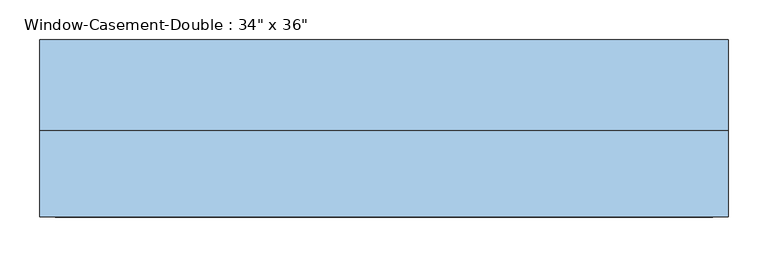
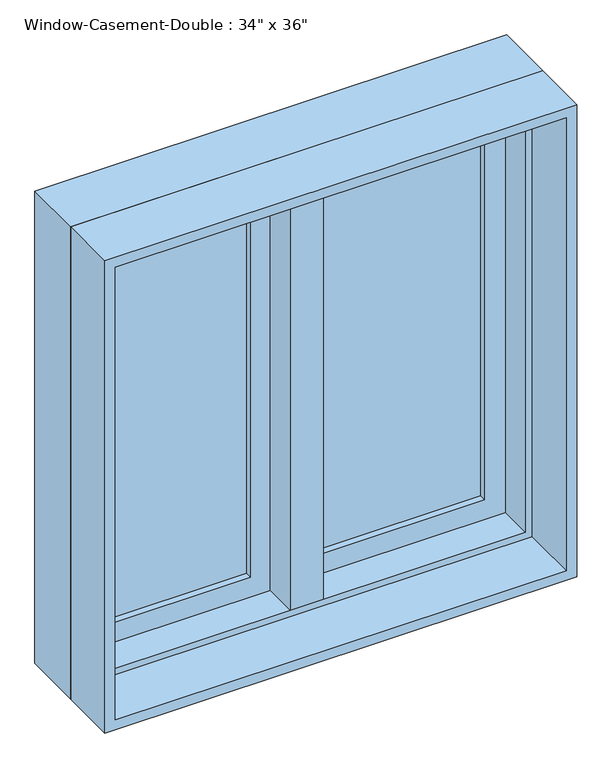
"""IFC4 building model written with IfcOpenShell, lengths in millimetres: window geometry."""

from ifc_helpers import new_model, si_unit, frame, origin, place, context, project, spatial, polyline, outline, extrude, faceted_brep, source, transform, mapped, element, save


def window_c29befe5(model_context):
    return source(origin(), model_context, "Body", "SolidModel", [
        faceted_brep([(9.525, 120.65, 1816.1), (-9.525, 120.65, 1816.1), (-9.525, 69.85, 1816.1), (9.525, 69.85, 1816.1), (9.525, 120.65, 927.1), (9.525, 69.85, 927.1), (-9.525, 69.85, 927.1), (-9.525, 120.65, 927.1), (-9.525, 69.85, 946.15), (-9.525, 69.85, 1797.05), (-30.1625, 69.85, 946.15), (-30.1625, 69.85, 1797.05), (-30.1625, 6.35, 946.15), (-30.1625, 6.35, 1797.05), (30.1625, 6.35, 946.15), (30.1625, 6.35, 1797.05), (30.1625, 69.85, 946.15), (30.1625, 69.85, 1797.05), (9.525, 69.85, 946.15), (9.525, 69.85, 1797.05)], [[[0, 1, 2, 3]], [[4, 5, 6, 7]], [[1, 0, 4, 7]], [[2, 1, 7, 6, 8, 9]], [[9, 8, 10, 11]], [[11, 10, 12, 13]], [[13, 12, 14, 15]], [[15, 14, 16, 17]], [[17, 16, 18, 19]], [[0, 3, 19, 18, 5, 4]], [[18, 8, 6, 5]], [[9, 19, 3, 2]], [[8, 18, 16, 14, 12, 10]], [[19, 9, 11, 13, 15, 17]]]),
        extrude(outline(polyline([(-66.675, 101.6), (-66.675, 95.25), (-361.95, 95.25), (-361.95, 101.6), (-66.675, 101.6)])), frame((0.0, 0.0, 984.25), z_axis=(0.0, 0.0, 1.0), x_axis=(1.0, 0.0, 0.0)), (0.0, 0.0, 1.0), 774.7),
        extrude(outline(polyline([(-361.95, 82.55), (-361.95, 88.9), (-66.675, 88.9), (-66.675, 82.55), (-361.95, 82.55)])), frame((0.0, 0.0, 984.25), z_axis=(0.0, 0.0, 1.0), x_axis=(1.0, 0.0, 0.0)), (0.0, 0.0, 1.0), 774.7),
        extrude(outline(polyline([(361.95, 101.6), (361.95, 95.25), (66.675, 95.25), (66.675, 101.6), (361.95, 101.6)])), frame((0.0, 0.0, 984.25), z_axis=(0.0, 0.0, 1.0), x_axis=(1.0, 0.0, 0.0)), (0.0, 0.0, 1.0), 774.7),
        extrude(outline(polyline([(66.675, 82.55), (66.675, 88.9), (361.95, 88.9), (361.95, 82.55), (66.675, 82.55)])), frame((0.0, 0.0, 984.25), z_axis=(0.0, 0.0, 1.0), x_axis=(1.0, 0.0, 0.0)), (0.0, 0.0, 1.0), 774.7),
        extrude(outline(polyline([(1816.1, -419.1), (927.1, -419.1), (927.1, -9.525), (1816.1, -9.525), (1816.1, -419.1)]), holes=[polyline([(1758.95, -66.675), (984.25, -66.675), (984.25, -361.95), (1758.95, -361.95), (1758.95, -66.675)])]), frame((0.0, 69.85, 0.0), z_axis=(0.0, 1.0, 0.0), x_axis=(0.0, 0.0, 1.0)), (0.0, 0.0, 1.0), 44.45),
        extrude(outline(polyline([(927.1, 419.1), (1816.1, 419.1), (1816.1, 9.525), (927.1, 9.525), (927.1, 419.1)]), holes=[polyline([(984.25, 66.675), (1758.95, 66.675), (1758.95, 361.95), (984.25, 361.95), (984.25, 66.675)])]), frame((0.0, 69.85, 0.0), z_axis=(0.0, 1.0, 0.0), x_axis=(0.0, 0.0, 1.0)), (0.0, 0.0, 1.0), 44.45),
        extrude(outline(polyline([(1828.8, -431.8), (914.4, -431.8), (914.4, 431.8), (1828.8, 431.8), (1828.8, -431.8)]), holes=[polyline([(1809.75, 412.75), (933.45, 412.75), (933.45, -412.75), (1809.75, -412.75), (1809.75, 412.75)])]), frame((0.0, -101.6, 0.0), z_axis=(0.0, 1.0, 0.0), x_axis=(0.0, 0.0, 1.0)), (0.0, 0.0, 1.0), 107.95),
        faceted_brep([(400.05, 69.85, 1797.05), (400.05, 6.35, 1797.05), (-400.05, 6.35, 1797.05), (-400.05, 69.85, 1797.05), (419.1, 120.65, 1816.1), (419.1, 69.85, 1816.1), (-419.1, 69.85, 1816.1), (-419.1, 120.65, 1816.1), (431.8, 6.35, 1828.8), (431.8, 120.65, 1828.8), (-431.8, 120.65, 1828.8), (-431.8, 6.35, 1828.8), (-400.05, 6.35, 946.15), (-400.05, 69.85, 946.15), (-419.1, 69.85, 927.1), (-419.1, 120.65, 927.1), (-431.8, 120.65, 914.4), (-431.8, 6.35, 914.4), (400.05, 6.35, 946.15), (400.05, 69.85, 946.15), (419.1, 69.85, 927.1), (419.1, 120.65, 927.1), (431.8, 120.65, 914.4), (431.8, 6.35, 914.4)], [[[0, 1, 2, 3]], [[4, 5, 6, 7]], [[8, 9, 10, 11]], [[3, 2, 12, 13]], [[7, 6, 14, 15]], [[11, 10, 16, 17]], [[13, 12, 18, 19]], [[15, 14, 20, 21]], [[17, 16, 22, 23]], [[11, 17, 23, 8], [1, 18, 12, 2]], [[19, 18, 1, 0]], [[5, 20, 14, 6], [3, 13, 19, 0]], [[21, 20, 5, 4]], [[23, 22, 9, 8]], [[9, 22, 16, 10], [7, 15, 21, 4]]]),
    ])


if __name__ == "__main__":
    model = new_model("IFC4")
    model_context = context("Model", 3, world=origin())
    ifc_project = project(units=[si_unit("LENGTHUNIT", "METRE", prefix="MILLI")], contexts=[model_context])
    site = spatial("IfcSite", under=ifc_project)
    building = spatial("IfcBuilding", under=site)
    placement = place(None, origin())
    window_shape = window_c29befe5(model_context)
    element("IfcWindow", 1, ObjectType="Window-Casement-Double : 34\" x 36\"", at=placement, inside=building, context=model_context, shape_type="MappedRepresentation", body=[
        mapped(window_shape, transform((0.0, 0.0, 0.0), x_axis=(1.0, 0.0, 0.0), y_axis=(0.0, 1.0, 0.0), z_axis=(0.0, 0.0, 1.0))),
    ])
    save(model, "model.ifc")

# Revit data of these elements
# Type "Window-Casement-Double : 34\" x 36\""
#   Type Mark = "14"
#   Fire Rating = "0.5h"
#   Assembly Code = "B2020100"
#   Analytic Construction = "Double glazing - domestic"
#   Frame Extension [instance default] = 0' - 0 1/4"
#   Window Inset [instance default] = 0' - 0"
#   Wall Thickness [instance default] = 0' - 6"
#   Interior Wall Closure [instance default] = 0' - 2 1/4"
#   Half Width = 1' - 5"
#   Visual Light Transmittance = 0.81
#   Thermal Resistance (R) = 1.8146 (h·ft²·°F)/BTU
#   Solar Heat Gain Coefficient = 0.76
#   Rough Width = 2' - 10 1/2"
#   Rough Height = 3' - 0 1/2"
#   Height = 3' - 0"
#   Heat Transfer Coefficient (U) = 0.5511 BTU/(h·ft²·°F)
#   Exterior Wall Closure [instance default] = 0' - 1 1/4"
#   Extension Jamb [instance default] = 0' - 2 1/4"
#   Default Sill Height = 3' - 0"
#   Width = 2' - 10"
#   Define Thermal Properties by = 0
#   Muntin Visibility = yes
#   Interior Trim Visibility [instance default] = yes
#   Exterior Trim Visibility [instance default] = yes
#   Extension Jamb Visibility [instance default] = yes
#   Interior Trim Material = Wood - Stained
#   Muntin Pattern = Muntin Pattern_2x2 : Muntin Pattern_2x2
#   Interior Trim = Trim-Window-Interior-Flat : Picture Frame
#   Interior Frame Material = Wood - Stained
#   Glass Panel Material = Glass
#   Exterior Trim Material = Clad - White
#   Exterior Trim = Trim-Window-Exterior-Flat : with Sill
#   Exterior Frame Material = Clad - White
#   Wall Closure = (empty or 0)
# Element 1 (IfcWindow, "Window-Casement-Double : 34\" x 36\"")
#   Wall Thickness = 0' - 8"
#   Extension Jamb = 0' - 4 1/4"
#   Materials on its faces: "Wood - Stained", "Glass", "Clad - White"
# Materials
#   "Wood - Stained": class "Wood", colour RGB 224 178 126, transparency 0, Cost = 0
#   "Glass": class "Glass", colour RGB 0 128 192, transparency 0.75, Description = "Soda Lime Glass", Cost = 0
#   "Clad - White": class "Wood", colour RGB 242 242 238, transparency 0, Cost = 0
